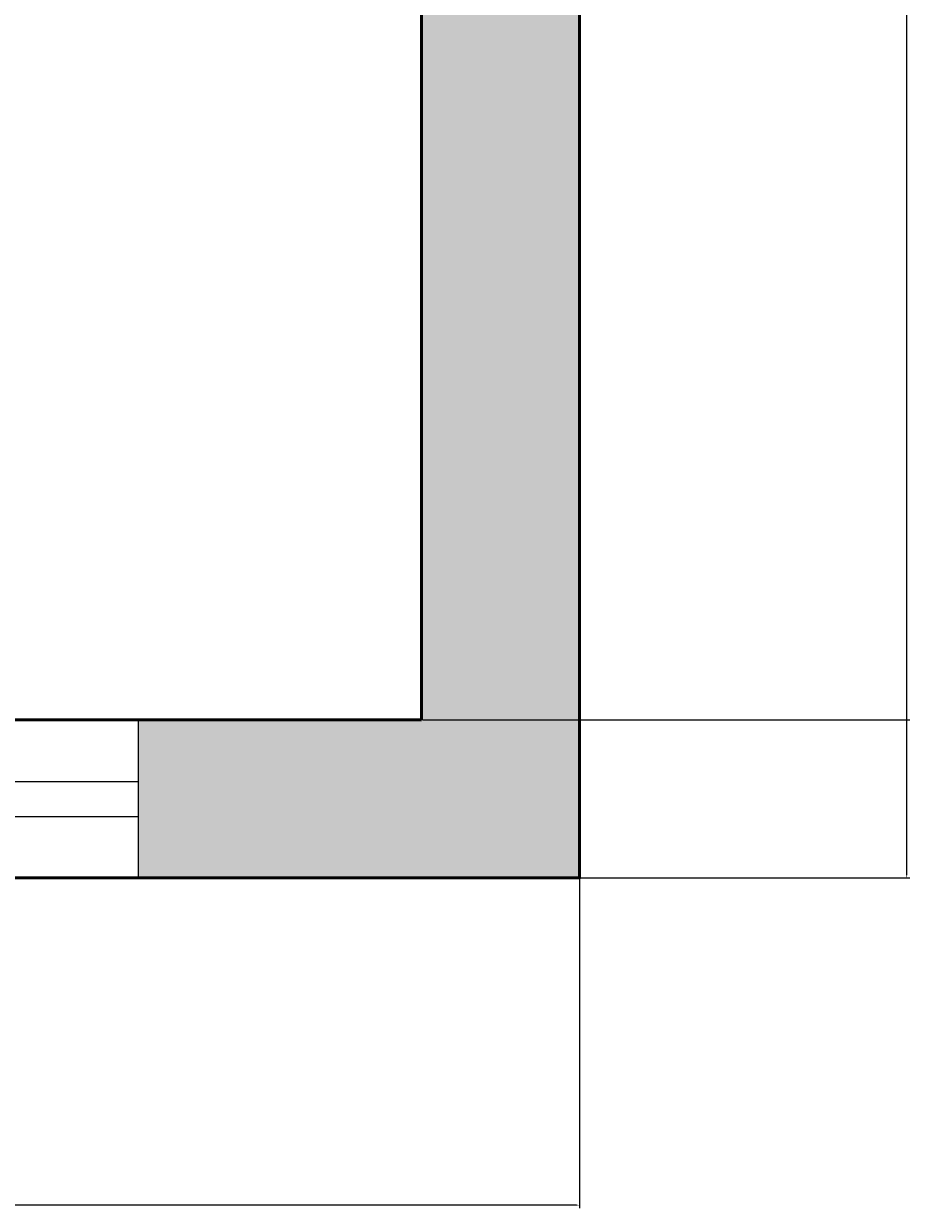
# Model space of a CAD drawing. Units: inches. Extents: x 2231 to 2461, y 2045 to 2455.
# Tile 22 of 95: x 2410 to 2461, y 2045 to 2112. Entities that reach past the tile are written whole.
import ezdxf

# ---------------------------------------------------------------- set-up
doc = ezdxf.new("R2010")
doc.units = ezdxf.units.IN
for name, color, linetype, lineweight in [('A-ANNO-DIMS', 2, 'Continuous', 18), ('A-GLAZ', 4, 'Continuous', 18), ('A-WALL', 7, 'Continuous', 50)]:
    doc.layers.add(name, color=color, linetype=linetype, lineweight=lineweight)
doc.layers.add('A-WALL-PATT', color=18, linetype='Continuous', lineweight=13, true_color=0x000000)
doc.styles.get("Standard").update_dxf_attribs({"font": 'arial.ttf'})
doc.dimstyles.get("Standard").update_dxf_attribs({"dimtxt": 0.18, "dimasz": 0.18, "dimexe": 0.18, "dimexo": 0.0625, "dimgap": 0.09, "dimtad": 0, "dimtih": 1, "dimtoh": 1, "dimdec": 4, "dimzin": 0, "dimdsep": 46, "dimtxsty": 'Standard', "dimcen": 0.09, "dimadec": 0, "dimazin": 0, "dimtfac": 1, "dimtdec": 4, "dimtofl": 0, "dimtmove": 0, "dimatfit": 3, "dimfxl": 1, "dimtolj": 1, "dimtzin": 0, "dimarcsym": 0})

# ---------------------------------------------------------------- blocks, each defined once
blk = doc.blocks.new('WIN-48IN')
for p, q in [((0, 0), (0, 9)), ((48, 9), (48, 0)), ((0, 5.5), (48, 5.5)), ((0, 3.5), (48, 3.5))]:
    blk.add_line(p, q)
blk = doc.blocks.new('*D33')
at = {"layer": 'A-ANNO-DIMS', "color": 0, "lineweight": -2, "transparency": 16777216}
for p, q in [((2249.794, 2063.77), (2249.794, 2045.02)), ((2441.794, 2063.77), (2441.794, 2045.02)), ((2249.974, 2045.2), (2345.514, 2045.2)), ((2441.614, 2045.2), (2346.073, 2045.2))]:
    blk.add_line(p, q, dxfattribs=at)
at = {"layer": 'A-ANNO-DIMS', "color": 0, "transparency": 16777216}
for points in [[(2249.974, 2045.23), (2249.974, 2045.17), (2249.794, 2045.2)], [(2441.614, 2045.23), (2441.614, 2045.17), (2441.794, 2045.2)]]:
    blk.add_solid(points, dxfattribs=at)
at = {"layer": 'Defpoints', "color": 0, "transparency": 16777216}
for p in [(2249.794, 2063.833), (2441.794, 2063.833), (2249.794, 2045.2)]:
    blk.add_point(p, dxfattribs=at)
at = {"layer": 'A-ANNO-DIMS', "color": 0, "transparency": 16777216, "insert": (2345.794, 2045.2), "char_height": 0.18, "attachment_point": 5}
blk.add_mtext('\\A1;192', dxfattribs=at)
blk = doc.blocks.new('*D34')
at = {"layer": 'A-ANNO-DIMS', "color": 0, "lineweight": -2, "transparency": 16777216}
for p, q in [((2441.856, 2435.833), (2460.606, 2435.833)), ((2460.426, 2435.653), (2460.426, 2250.015)), ((2460.426, 2064.013), (2460.426, 2249.651)), ((2441.856, 2063.833), (2460.606, 2063.833))]:
    blk.add_line(p, q, dxfattribs=at)
at = {"layer": 'A-ANNO-DIMS', "color": 0, "transparency": 16777216}
for points in [[(2460.396, 2435.653), (2460.456, 2435.653), (2460.426, 2435.833)], [(2460.396, 2064.013), (2460.456, 2064.013), (2460.426, 2063.833)]]:
    blk.add_solid(points, dxfattribs=at)
at = {"layer": 'Defpoints', "color": 0, "transparency": 16777216}
for p in [(2441.794, 2435.833), (2460.426, 2435.833), (2441.794, 2063.833)]:
    blk.add_point(p, dxfattribs=at)
at = {"layer": 'A-ANNO-DIMS', "color": 0, "transparency": 16777216, "insert": (2460.426, 2249.833), "char_height": 0.18, "attachment_point": 5}
blk.add_mtext('\\A1;372', dxfattribs=at)
blk = doc.blocks.new('*D41')
at = {"layer": 'A-ANNO-DIMS', "color": 0, "lineweight": -2, "transparency": 16777216}
for p, q in [((2432.856, 2182.833), (2460.606, 2182.833)), ((2460.426, 2182.653), (2460.426, 2128.015)), ((2460.426, 2073.013), (2460.426, 2127.651)), ((2432.856, 2072.833), (2460.606, 2072.833))]:
    blk.add_line(p, q, dxfattribs=at)
at = {"layer": 'A-ANNO-DIMS', "color": 0, "transparency": 16777216}
for points in [[(2460.396, 2182.653), (2460.456, 2182.653), (2460.426, 2182.833)], [(2460.396, 2073.013), (2460.456, 2073.013), (2460.426, 2072.833)]]:
    blk.add_solid(points, dxfattribs=at)
at = {"layer": 'Defpoints', "color": 0, "transparency": 16777216}
for p in [(2432.794, 2182.833), (2460.426, 2182.833), (2432.794, 2072.833)]:
    blk.add_point(p, dxfattribs=at)
at = {"layer": 'A-ANNO-DIMS', "color": 0, "transparency": 16777216, "insert": (2460.426, 2127.833), "char_height": 0.18, "attachment_point": 5}
blk.add_mtext('\\A1;110', dxfattribs=at)

msp = doc.modelspace()

# ---------------------------------------------------------------- hatches: boundary and pattern name
at = {"layer": 'A-WALL-PATT'}
h = msp.add_hatch(color=256, dxfattribs=at)
h.dxf.hatch_style = 1
h.paths.add_polyline_path([(2441.7935, 2269.1535), (2432.7935, 2269.1535), (2432.7935, 2186.8328), (2396.7935, 2186.8328), (2396.7935, 2286.8328), (2394.7935, 2286.8328), (2394.7935, 2186.8328), (2334.7935, 2186.8328), (2334.7935, 2182.8328), (2432.7935, 2182.8328), (2432.7935, 2072.8328), (2416.6639, 2072.8328), (2416.6639, 2063.8328), (2441.7935, 2063.8328)])
h.paths.add_polyline_path([(2368.6639, 2072.8328), (2367.04, 2072.8328), (2330.7942, 2072.8328), (2330.7397, 2063.8328), (2368.6639, 2063.8328)])
h.paths.add_polyline_path([(2300.7392, 2068.3328), (2300.7392, 2072.8328), (2298.7935, 2072.8328), (2294.7935, 2072.8328), (2258.7935, 2072.8328), (2258.7935, 2120.8328), (2294.7935, 2120.8328), (2298.7935, 2120.8328), (2298.7935, 2128.8328), (2294.7935, 2128.8328), (2294.7935, 2124.8328), (2258.7935, 2124.8328), (2258.7935, 2182.8328), (2294.7935, 2182.8328), (2294.7935, 2174.8328), (2298.7935, 2174.8328), (2298.7935, 2182.8328), (2304.7935, 2182.8328), (2304.7935, 2186.8328), (2258.7935, 2186.8328), (2258.7935, 2221.999), (2249.7935, 2221.999), (2249.7935, 2063.8328), (2300.7392, 2063.8328)])
h.paths.add_polyline_path([(2391.9338, 2435.8328), (2333.82, 2435.8328), (2333.82, 2426.8328), (2368.7935, 2426.8328), (2368.7935, 2374.9508), (2368.7935, 2370.8328), (2372.3935, 2370.8328), (2372.7935, 2370.8328), (2372.7935, 2426.8328), (2391.9338, 2426.8328)])
h.paths.add_polyline_path([(2441.7935, 2435.8328), (2415.9338, 2435.8328), (2415.9338, 2426.8328), (2432.7935, 2426.8328), (2432.7935, 2334.8328), (2372.7935, 2334.8328), (2372.7935, 2346.8328), (2368.7935, 2346.8328), (2368.7935, 2306.8328), (2360.7935, 2306.8328), (2360.7935, 2302.8328), (2368.7935, 2302.8328), (2372.7935, 2302.8328), (2372.7935, 2330.8328), (2432.7935, 2330.8328), (2432.7935, 2317.1535), (2441.7935, 2317.1535)])
h.paths.add_polyline_path([(2285.82, 2435.8328), (2249.7935, 2435.8328), (2249.7935, 2269.999), (2258.7935, 2269.999), (2258.7935, 2302.8328), (2318.8168, 2302.8328), (2330.7935, 2302.8328), (2330.7935, 2306.8328), (2258.7935, 2306.8328), (2258.7935, 2426.8328), (2285.82, 2426.8328)])

# ---------------------------------------------------------------- linework, layer by layer
at = {"layer": 'A-WALL'}
for p, q in [((2432.7935, 2182.8328), (2432.7935, 2072.8328)), ((2432.7935, 2072.8328), (2330.7942, 2072.8328))]:
    msp.add_line(p, q, dxfattribs=at)
msp.add_lwpolyline([(2300.7392, 2063.8328), (2249.7935, 2063.8328), (2249.7935, 2435.8328), (2441.7935, 2435.8328), (2441.7935, 2063.8328), (2330.7397, 2063.8328)], dxfattribs=at)

# ---------------------------------------------------------------- block references
at = {"layer": 'A-GLAZ'}
msp.add_blockref('WIN-48IN', (2368.6639, 2063.833), dxfattribs=at)

# ---------------------------------------------------------------- dimensions: what is measured, and where the dimension line sits
at = {"layer": 'A-ANNO-DIMS'}
for base, p1, p2, angle, picture, middle in [((2460.426, 2435.8328), (2441.7935, 2063.8328), (2441.7935, 2435.8328), 90, '*D34', (2460.426, 2249.8328)), ((2460.426, 2182.8328), (2432.7935, 2072.8328), (2432.7935, 2182.8328), 90, '*D41', (2460.426, 2127.8328)), ((2249.7935, 2045.2003), (2441.7935, 2063.8328), (2249.7935, 2063.8328), 180, '*D33', (2345.7935, 2045.2003))]:
    dim = msp.add_linear_dim(base=base, p1=p1, p2=p2, angle=angle, dimstyle='Standard', override={"dimdec": 0, "dimlfac": 1, "dimrnd": 0, "dimzin": 0, "dimdsep": 46, "dimlunit": 2}, dxfattribs=at)
    dim.commit()
    dim.dimension.update_dxf_attribs({"geometry": picture, "text_midpoint": middle})

doc.saveas('drawing.dxf')
